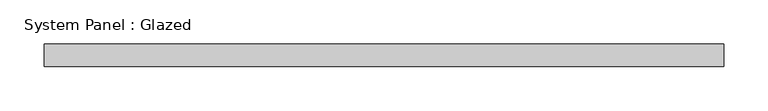
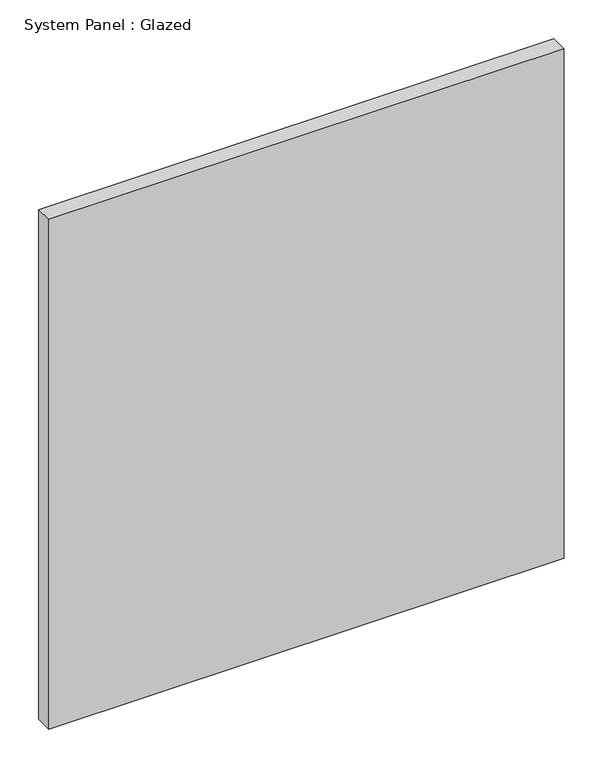
"""IFC4 building model written with IfcOpenShell, lengths in millimetres: plate geometry, System Panel : Glazed."""

from ifc_helpers import new_model, si_unit, origin, origin_with_axes, place, context, project, spatial, polyline, outline, extrude, source, transform, mapped, element, save


def system_panel_glazed_75f85cfe(model_context):
    return source(origin(), model_context, "Body", "SweptSolid", [
        extrude(outline(polyline([(383.50825, 19.05), (-383.50825, 19.05), (-383.50825, 44.45), (383.50825, 44.45), (383.50825, 19.05)])), origin_with_axes(), (0.0, 0.0, 1.0), 801.9415),
    ])


if __name__ == "__main__":
    model = new_model("IFC4")
    model_context = context("Model", 3, world=origin())
    ifc_project = project(units=[si_unit("LENGTHUNIT", "METRE", prefix="MILLI")], contexts=[model_context])
    site = spatial("IfcSite", under=ifc_project)
    building = spatial("IfcBuilding", under=site)
    placement = place(None, origin())
    system_panel_glazed_shape = system_panel_glazed_75f85cfe(model_context)
    element("IfcPlate", 1, ObjectType="System Panel : Glazed", at=placement, inside=building, context=model_context, shape_type="MappedRepresentation", body=[
        mapped(system_panel_glazed_shape, transform((0.0, 0.0, 0.0), x_axis=(1.0, 0.0, 0.0), y_axis=(0.0, 1.0, 0.0), z_axis=(0.0, 0.0, 1.0))),
    ])
    save(model, "model.ifc")

# Revit data of these elements
# Type "System Panel : Glazed"
#   Construction Type Id = "GSP4R"
#   Analytic Construction = "1/8 in Pilkington single glazing"
#   Visual Light Transmittance = 0.9
#   Solar Heat Gain Coefficient = 0.86
#   Heat Transfer Coefficient (U) = 1.18115 BTU/(h·ft²·°F)
#   Define Thermal Properties by = 1
# Element 1 (IfcPlate, "System Panel : Glazed")
#   Materials on its faces: "Glass"
# Materials
#   "Glass": class "Glass", colour RGB 0 128 192, transparency 0.75, Description = "Soda Lime Glass", Cost = 0
